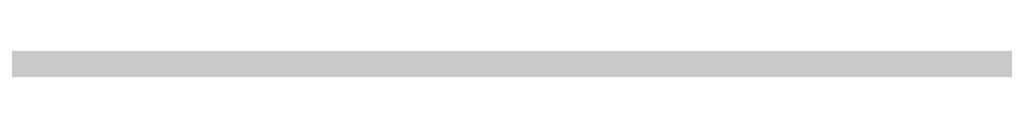
# Model space of a CAD drawing. Units: inches. Extents: x 2091 to 2899, y 967 to 2217.
# Tile 183 of 256: x 2203.16122 to 2203.18039, y 1152.24727 to 1152.24748. Entities that reach past the tile are written whole.
import ezdxf

# ---------------------------------------------------------------- set-up
doc = ezdxf.new("R2010")
doc.units = ezdxf.units.IN
doc.layers.add('A-WALL-PATT', color=141, linetype='Continuous', lineweight=13, true_color=0xadddf7)

msp = doc.modelspace()

# ---------------------------------------------------------------- hatches: boundary and pattern name
at = {"layer": 'A-WALL-PATT'}
h = msp.add_hatch(color=256, dxfattribs=at)
h.dxf.hatch_style = 1
h.paths.add_polyline_path([(2803.143603, 2050.919059), (2203.143603, 2050.919059), (2203.143603, 1090.919059), (2803.143603, 1090.919059)])
h.paths.add_polyline_path([(2635.79885, 1147.540465), (2674.524052, 1147.540465, 0.376086), (2678.529665, 1152.880202), (2678.529665, 1159.556473, 0.333335), (2674.524319, 1163.561846), (2674.524319, 1163.56185), (2674.524319, 1192.93439), (2635.805971, 1192.93439), (2597.087622, 1192.93439), (2597.087622, 1163.561846, 0.333335), (2593.082276, 1159.556473), (2593.082276, 1152.880202, 0.376086), (2597.087889, 1147.540465)], flags=0)
h.paths.add_polyline_path([(2436.010433, 1278.240778, 0.000483), (2435.952643, 1278.215027, -0.001328), (2435.935625, 1278.111693, -0.001711), (2436.11644, 1278.040758, 0.002185)], flags=0)
h.paths.add_polyline_path([(2794.143603, 1143.419059), (2794.143603, 1347.419059), (2543.370171, 1347.419059), (2543.370171, 1351.919059), (2794.143603, 1351.919059), (2794.143603, 1392.713555), (2793.947398, 1392.713555), (2793.947398, 1473.5369), (2794.143603, 1473.5369), (2794.143603, 1531.919059), (2650.143603, 1531.919059), (2650.143603, 1536.419059), (2794.143603, 1536.419059), (2794.143603, 1692.419059), (2609.375609, 1692.419059), (2609.375609, 1644.419059), (2604.875609, 1644.419059), (2604.875609, 1744.919059), (2609.375609, 1744.919059), (2609.375609, 1696.919059), (2794.143603, 1696.919059), (2794.143603, 1780.919059), (2609.643603, 1780.919059), (2493.875609, 1780.919059), (2493.875609, 1785.419059), (2609.643603, 1785.419059), (2794.143603, 1785.419059), (2794.143603, 1847.938821), (2793.951222, 1847.938821), (2793.951222, 1928.762166), (2794.143603, 1928.762166), (2794.143603, 1941.419059), (2614.143603, 1941.419059), (2614.143603, 1821.419059), (2609.643603, 1821.419059), (2609.643603, 1941.419059), (2392.143603, 1941.419059), (2392.143603, 1819.919059), (2387.643603, 1819.919059), (2387.643603, 1941.419059), (2212.143603, 1941.419059), (2212.143603, 1783.919059), (2392.143603, 1783.919059), (2392.143603, 1780.919059), (2212.143603, 1780.919059), (2212.143603, 1629.419059), (2387.643603, 1629.419059), (2387.643603, 1744.919059), (2392.143603, 1744.919059), (2392.143603, 1627.919059), (2317.143603, 1627.919059), (2317.143603, 1551.419059), (2317.143603, 1536.419059), (2459.383591, 1536.419059), (2459.383591, 1602.39648), (2463.883591, 1602.39648), (2463.883591, 1531.919059), (2456.643603, 1531.919059), (2456.643603, 1529.919059), (2452.143603, 1529.919059), (2452.143603, 1531.919059), (2312.643603, 1531.919059), (2312.643603, 1551.419059), (2306.143603, 1551.419059), (2306.143603, 1555.919059), (2308.143603, 1555.919059), (2308.143603, 1551.419059), (2312.643603, 1551.419059), (2312.643603, 1627.919059), (2212.143603, 1627.919059), (2212.143603, 1555.919059), (2270.143603, 1555.919059), (2270.143603, 1551.419059), (2212.143603, 1551.419059), (2212.143603, 1351.919059), (2272.143603, 1351.919059), (2272.143603, 1347.419059), (2212.143603, 1347.419059), (2212.143603, 1275.419059), (2308.143603, 1275.419059), (2308.143603, 1351.919059), (2452.143603, 1351.919059), (2452.143603, 1493.919059), (2456.643603, 1493.919059), (2456.643603, 1347.419059), (2312.643603, 1347.419059), (2312.643603, 1270.919059), (2212.143603, 1270.919059), (2212.143603, 1099.919059), (2281.237523, 1099.919059), (2282.871041, 1110.913803), (2282.008341, 1116.996603), (2278.557741, 1121.420403), (2268.205641, 1128.056203), (2272.087641, 1128.056203), (2273.812941, 1131.927003), (2279.420341, 1134.691903), (2285.027841, 1135.244903), (2287.615841, 1137.456803), (2288.047141, 1138.009803), (2289.341141, 1140.774703), (2291.066541, 1139.668703), (2292.360541, 1135.244903), (2295.379841, 1136.903803), (2296.242541, 1135.797903), (2297.105241, 1133.033003), (2300.124641, 1138.009803), (2303.143941, 1138.009803), (2304.437941, 1135.797903), (2303.143941, 1133.586003), (2306.594641, 1134.691903), (2307.888741, 1133.033003), (2310.908041, 1135.244903), (2313.927441, 1134.138903), (2315.62686, 1132.427102), (2308.320041, 1117.549603), (2290.203841, 1109.807903), (2288.909841, 1103.172103), (2289.272309, 1099.919059), (2434.918227, 1099.919059), (2431.593227, 1124.788059), (2429.930227, 1169.553059), (2430.927185, 1240.519694), (2435.658926, 1238.186126), (2437.135227, 1196.554059), (2438.798227, 1143.973059), (2442.678227, 1111.998059), (2446.558227, 1099.919059), (2794.143603, 1099.919059), (2794.143603, 1138.919059), (2548.032447, 1138.919059), (2548.032447, 1143.419059), (2548.032447, 1148.819059), (2546.668457, 1148.031559), (2528.685692, 1179.178622, 0.256256), (2512.032447, 1148.819059), (2512.032447, 1143.419059), (2512.032447, 1138.919059), (2507.532447, 1138.919059), (2507.532447, 1143.419059), (2507.532447, 1148.819059, 0.256256), (2490.879202, 1179.178622), (2472.896437, 1148.031559), (2471.532447, 1148.819059), (2471.532447, 1143.419059), (2467.032447, 1143.419059), (2467.032447, 1269.945786, 0.039061), (2460.909987, 1273.580059), (2467.032447, 1273.580059), (2467.032447, 1286.325364, 0.014511), (2465.216194, 1286.761905), (2467.032447, 1287.052576), (2467.032447, 1323.419059), (2471.532447, 1323.419059), (2471.532447, 1148.819059), (2489.532447, 1179.995973), (2490.896437, 1179.208473), (2490.879202, 1179.178622, -0.256256), (2507.532447, 1148.819059), (2507.532447, 1143.419059), (2512.032447, 1143.419059), (2512.032447, 1148.819059, -0.256256), (2528.685692, 1179.178622), (2528.668457, 1179.208473), (2530.032447, 1179.995973), (2548.032447, 1148.819059), (2548.032447, 1143.419059)], flags=16)
h.paths.add_polyline_path([(2607.768546, 1200.945083), (2607.768546, 1265.030625), (2597.087622, 1281.052011), (2619.784585, 1281.052011), (2627.795278, 1337.12686), (2635.79885, 1337.12686), (2643.816663, 1337.12686), (2651.827356, 1281.052011), (2674.524319, 1281.052011), (2663.843395, 1265.030625), (2663.843395, 1200.945083), (2635.805971, 1200.945083)], flags=0)
edge = h.paths.add_edge_path(flags=0)
edge.add_ellipse((13303.896215, 1272.998725), major_axis=(-10595.31304, 0.000001), ratio=0.842303870086, start_angle=0.6282372191, end_angle=0.6465540999, ccw=False)
edge.add_ellipse((2711.70045, 1156.852678), major_axis=(2.219769, 0), ratio=0.84230387, start_angle=111.535244, end_angle=180.628237, ccw=False)
edge.add_ellipse((13303.156292, 1272.998725), major_axis=(-10593.026306, 0), ratio=0.842303869544, start_angle=0.5282714718, end_angle=0.6465540971, ccw=False)
edge.add_line((2710.764596, 1175.333295), (2710.129986, 1175.333295))
edge.add_ellipse((2710.129986, 1176.579775), major_axis=(1.479846, 0), ratio=0.84230387, start_angle=180, end_angle=270, ccw=False)
edge.add_line((2708.65014, 1176.579775), (2708.65014, 1200.782914))
edge.add_ellipse((2710.129986, 1200.782914), major_axis=(1.479846, 0), ratio=0.84230387, start_angle=90, end_angle=180, ccw=False)
edge.add_line((2710.129986, 1202.029394), (2710.465075, 1202.029394))
edge.add_ellipse((13303.156292, 1272.998725), major_axis=(-10593.026306, 0), ratio=0.842303869544, start_angle=-0.0902290886, end_angle=0.3838667788, ccw=False)
edge.add_ellipse((2710.129986, 1290.927031), major_axis=(-1.479846, 0), ratio=0.84230387, start_angle=0, end_angle=90, ccw=False)
edge.add_line((2708.65014, 1290.927031), (2708.65014, 1315.13017))
edge.add_ellipse((2710.129986, 1315.13017), major_axis=(-1.479846, 0), ratio=0.84230387, start_angle=-90, end_angle=0, ccw=False)
edge.add_line((2710.129986, 1316.37665), (2710.706314, 1316.37665))
edge.add_ellipse((3238.40172, 1296.289566), major_axis=(528.234, 0), ratio=0.8423038695, start_angle=176.34957241, end_angle=177.82004969, ccw=False)
edge.add_ellipse((2775.063043, 1071.450696), major_axis=(313.307761, 0), ratio=0.8423038695, start_angle=102.12596555, end_angle=103.78052899, ccw=False)
edge.add_ellipse((2775.063043, 1078.305698), major_axis=(-305.302891, 0), ratio=0.8423038695, start_angle=-79.790461, end_angle=-77.55537271, ccw=False)
edge.add_ellipse((2695.141767, 1541.975383), major_axis=(-250.960216, 0), ratio=0.8423038695, start_angle=99.25656601, end_angle=102.55493264)
edge.add_line((2741.410326, 1334.214255), (2747.132545, 1337.378477))
edge.add_ellipse((2747.538616, 1336.857478), major_axis=(-0.739923, 0), ratio=0.8423039, start_angle=270, end_angle=307.93313, ccw=False)
edge.add_ellipse((2747.538616, 1336.857478), major_axis=(-0.739923, 0), ratio=0.8423039, start_angle=232.06687, end_angle=270, ccw=False)
edge.add_line((2747.944687, 1337.378477), (2753.666906, 1334.214255))
edge.add_ellipse((2799.935466, 1541.975383), major_axis=(250.960216, 0), ratio=0.8423038695, start_angle=257.44506736, end_angle=260.74343399)
edge.add_ellipse((2720.014189, 1078.305698), major_axis=(305.302891, 0), ratio=0.8423038695, start_angle=77.55537271, end_angle=79.790461, ccw=False)
edge.add_ellipse((2720.014189, 1071.450696), major_axis=(-313.307761, 0), ratio=0.8423038695, start_angle=256.21947101, end_angle=257.87403445, ccw=False)
edge.add_ellipse((2256.675512, 1296.289566), major_axis=(-528.234, 0), ratio=0.8423038695, start_angle=182.17995031, end_angle=183.65042759, ccw=False)
edge.add_line((2784.370918, 1316.37665), (2784.947247, 1316.37665))
edge.add_ellipse((2784.947247, 1315.13017), major_axis=(1.479846, 0), ratio=0.84230387, start_angle=0, end_angle=90, ccw=False)
edge.add_line((2786.427093, 1315.13017), (2786.427093, 1290.927031))
edge.add_ellipse((2784.947247, 1290.927031), major_axis=(1.479846, 0), ratio=0.84230387, start_angle=270, end_angle=360, ccw=False)
edge.add_ellipse((-7808.07906, 1272.998725), major_axis=(10593.026306, 0), ratio=0.842303869544, start_angle=-0.3838667788, end_angle=0.0902290886, ccw=False)
edge.add_line((2784.612157, 1202.029394), (2784.947247, 1202.029394))
edge.add_ellipse((2784.947247, 1200.782914), major_axis=(1.479846, 0), ratio=0.84230387, start_angle=0, end_angle=90, ccw=False)
edge.add_line((2786.427093, 1200.782914), (2786.427093, 1176.579775))
edge.add_ellipse((2784.947247, 1176.579775), major_axis=(-1.479846, 0), ratio=0.84230387, start_angle=90, end_angle=180, ccw=False)
edge.add_line((2784.947247, 1175.333295), (2784.312636, 1175.333295))
edge.add_ellipse((-7808.07906, 1272.998725), major_axis=(10593.026306, 0), ratio=0.842303869544, start_angle=-0.6186431963, end_angle=-0.5282714718, ccw=False)
edge.add_ellipse((2783.376783, 1156.852678), major_axis=(-2.219769, 0), ratio=0.84230387, start_angle=179.371763, end_angle=248.464757, ccw=False)
edge.add_ellipse((-7808.818983, 1272.998725), major_axis=(-10595.31304, 0.000004), ratio=0.842303865762, start_angle=179.3534459226, end_angle=179.3717628034, ccw=False)
edge.add_ellipse((2780.297303, 1153.500793), major_axis=(-5.246426, 0), ratio=0.84230387, start_angle=90, end_angle=179.353446, ccw=False)
edge.add_line((2780.297303, 1149.081708), (2714.77993, 1149.081708))
edge.add_ellipse((2714.77993, 1153.500793), major_axis=(5.246426, 0), ratio=0.84230387, start_angle=180.646554, end_angle=270, ccw=False)
edge = h.paths.add_edge_path(flags=0)
edge.add_line((2718.187367, 1151.007833), (2718.187367, 1170.472364))
edge.add_ellipse((2721.14706, 1170.472364), major_axis=(-2.959692, 0), ratio=0.84230387, start_angle=-90, end_angle=0, ccw=False)
edge.add_line((2721.14706, 1172.965324), (2773.930173, 1172.965324))
edge.add_ellipse((2773.930173, 1170.472364), major_axis=(-2.959692, 0), ratio=0.84230387, start_angle=180, end_angle=270, ccw=False)
edge.add_line((2776.889865, 1170.472364), (2776.889865, 1151.007833))
edge.add_line((2776.889865, 1151.007833), (2718.187367, 1151.007833))
edge = h.paths.add_edge_path(flags=0)
edge.add_line((2718.187367, 1180.23415), (2718.187367, 1199.057834))
edge.add_ellipse((2747.538616, 1320.39864), major_axis=(147.017924, 0), ratio=0.8423038695, start_angle=256.40186531, end_angle=283.59813469)
edge.add_line((2776.889865, 1199.057834), (2776.889865, 1180.23415))
edge.add_ellipse((2747.538616, 1301.574956), major_axis=(147.017924, 0), ratio=0.8423038695, start_angle=256.40186531, end_angle=283.59813469, ccw=False)
edge = h.paths.add_edge_path(flags=0)
edge.add_ellipse((13303.156292, 1272.998725), major_axis=(-10591.54646, 0), ratio=0.842303869555, start_angle=0.0555943135, end_angle=0.3777641939, ccw=False)
edge.add_line((2711.616859, 1262.72171), (2715.667408, 1249.495396))
edge.add_ellipse((6413.891963, 1241.691919), major_axis=(-3698.236159, 0), ratio=0.84230386955, start_angle=-0.120897369, end_angle=0.364076349)
edge.add_line((2715.761038, 1218.192455), (2711.934307, 1203.167361))
edge = h.paths.add_edge_path(flags=0)
edge.add_line((2718.187367, 1251.074566), (2716.002485, 1267.450435))
edge.add_ellipse((2742.151175, 1202.18954), major_axis=(81.772585, 0), ratio=0.84230387, start_angle=94.27742096, end_angle=111.8349538, ccw=False)
edge.add_line((2737.009748, 1270.930626), (2758.067484, 1270.930626))
edge.add_ellipse((2752.926058, 1202.18954), major_axis=(81.772585, 0), ratio=0.84230387, start_angle=68.1650462, end_angle=85.72257904, ccw=False)
edge.add_line((2779.074747, 1267.450435), (2776.889865, 1251.074566))
edge.add_ellipse((2750.338059, 1187.885356), major_axis=(79.579664, 0), ratio=0.84230387, start_angle=67.20808512, end_angle=85.1299304)
edge.add_line((2756.034656, 1254.743656), (2739.042576, 1254.743656))
edge.add_ellipse((2744.739174, 1187.885356), major_axis=(79.579664, 0), ratio=0.84230387, start_angle=94.8700696, end_angle=112.79191488)
edge = h.paths.add_edge_path(flags=0)
edge.add_line((2783.142926, 1203.167361), (2779.316194, 1218.192455))
edge.add_ellipse((-918.81473, 1241.691919), major_axis=(3698.236159, 0), ratio=0.84230386955, start_angle=-0.364076349, end_angle=0.120897369)
edge.add_line((2779.409825, 1249.495396), (2783.460373, 1262.72171))
edge.add_ellipse((-7808.07906, 1272.998725), major_axis=(-10591.54646, 0), ratio=0.84230386954, start_angle=179.6222358061, end_angle=179.9444056865, ccw=False)
edge = h.paths.add_edge_path(flags=0)
edge.add_ellipse((2734.200892, 1286.69044), major_axis=(-0.356609, 6.340078), ratio=0.60383358, start_angle=89.0020143, end_angle=253.657408, ccw=False)
edge.add_line((2730.369001, 1286.541806), (2730.369001, 1301.35198))
edge.add_line((2730.369001, 1301.35198), (2735.913311, 1305.214803))
edge.add_ellipse((2736.384917, 1304.734561), major_axis=(0.739923, 0), ratio=0.8423039, start_angle=90, end_angle=134.480211, ccw=False)
edge.add_line((2736.384917, 1305.357801), (2738.032783, 1305.357801))
edge.add_line((2738.032783, 1305.357801), (2738.032783, 1307.707927))
edge.add_ellipse((2794.201642, 1307.707927), major_axis=(56.168859, 0), ratio=0.84230387, start_angle=150.5614304, end_angle=180, ccw=False)
edge.add_ellipse((2700.875591, 1307.707927), major_axis=(-56.168859, 0), ratio=0.84230387, start_angle=180, end_angle=209.4385696, ccw=False)
edge.add_line((2757.04445, 1307.707927), (2757.04445, 1305.357801))
edge.add_line((2757.04445, 1305.357801), (2758.692316, 1305.357801))
edge.add_ellipse((2758.692316, 1304.734561), major_axis=(-0.739923, 0), ratio=0.8423039, start_angle=225.519789, end_angle=270, ccw=False)
edge.add_line((2759.163922, 1305.214803), (2764.708231, 1301.35198))
edge.add_line((2764.708231, 1301.35198), (2764.708231, 1286.541806))
edge.add_ellipse((2760.87634, 1286.69044), major_axis=(0.356609, 6.340078), ratio=0.60383358, start_angle=106.342592, end_angle=270.9979857, ccw=False)
edge.add_line((2757.04445, 1285.79709), (2757.04445, 1307.707927))
edge.add_ellipse((2700.875591, 1307.707927), major_axis=(-56.168859, 0), ratio=0.84230387, start_angle=180, end_angle=209.4385696)
edge.add_ellipse((2794.201642, 1307.707927), major_axis=(56.168859, 0), ratio=0.84230387, start_angle=150.5614304, end_angle=180)
edge.add_line((2738.032783, 1307.707927), (2738.032783, 1285.79709))
h.paths.add_polyline_path([(2417.812273, 1104.449704), (2413.492273, 1102.529704), (2410.612273, 1103.969704), (2409.172273, 1106.369704), (2407.252273, 1107.329704), (2406.292273, 1109.729704), (2405.332273, 1114.049704), (2405.332273, 1117.889704), (2406.292273, 1120.129704), (2407.252273, 1119.809704), (2408.848322, 1118.327658), (2410.173945, 1119.42417), (2410.211273, 1120.405704), (2411.040731, 1121.419054), (2410.699273, 1119.858704), (2410.173945, 1119.42417), (2410.088452, 1117.176109), (2411.132836, 1116.206324), (2413.972273, 1119.329704), (2416.852273, 1120.769704), (2416.869721, 1120.798784), (2417.035071, 1119.405116), (2417.896213, 1118.143384), (2418.292273, 1118.369704), (2419.544447, 1120.039269), (2419.360915, 1118.387487), (2419.032108, 1119.356151), (2418.398939, 1118.511926), (2419.252273, 1114.529704), (2418.794091, 1107.198795)], flags=0)
h.paths.add_polyline_path([(2508.870171, 1347.419059), (2508.370171, 1347.419059), (2508.370171, 1351.919059), (2508.870171, 1351.919059)], flags=0)
h.paths.add_polyline_path([(2473.370171, 1347.419059), (2472.370171, 1347.419059), (2467.870171, 1347.419059), (2467.870171, 1455.419059), (2472.370171, 1455.419059), (2472.370171, 1352.419059), (2473.370171, 1352.419059)], flags=0)
h.paths.add_polyline_path([(2352.106244, 1217.446197), (2349.226244, 1218.886197), (2347.786244, 1221.286197), (2345.866244, 1222.246197), (2344.906244, 1224.646197), (2343.946244, 1228.966197), (2343.946244, 1232.806197), (2344.906244, 1235.046197), (2345.866244, 1234.726197), (2347.462293, 1233.244152), (2348.787916, 1234.340663), (2348.825244, 1235.322197), (2349.654702, 1236.335547), (2349.313244, 1234.775197), (2348.787916, 1234.340663), (2348.702423, 1232.092603), (2349.746807, 1231.122817), (2352.586244, 1234.246197), (2355.466244, 1235.686197), (2355.483692, 1235.715277), (2355.649043, 1234.321609), (2356.510185, 1233.059877), (2356.906244, 1233.286197), (2358.158418, 1234.955762), (2357.974887, 1233.30398), (2357.646079, 1234.272644), (2357.012911, 1233.428419), (2357.866244, 1229.446197), (2357.408062, 1222.115288), (2356.426244, 1219.366197)], flags=0)
h.paths.add_polyline_path([(2348.2968, 1112.22442), (2347.0138, 1112.31042), (2345.5298, 1114.12742), (2345.7318, 1115.85842), (2346.8118, 1116.98242), (2346.8118, 1114.64642), (2345.8668, 1114.21442), (2346.8798, 1114.30042)], flags=0)
h.paths.add_polyline_path([(2347.0138, 1110.92642), (2346.2718, 1110.49342), (2346.6098, 1111.18642)], flags=0)
h.paths.add_polyline_path([(2345.8668, 1118.19442), (2345.5298, 1117.32942), (2343.7078, 1118.02142), (2344.3828, 1118.62642)], flags=0)
h.paths.add_polyline_path([(2346.6768, 1109.28242), (2346.0698, 1108.07142), (2345.8668, 1110.06142)], flags=0)
h.paths.add_polyline_path([(2345.0568, 1119.75142), (2343.6398, 1119.75142), (2343.9778, 1121.13542)], flags=0)
h.paths.add_polyline_path([(2345.2598, 1116.55042), (2345.1248, 1115.85842), (2344.9218, 1115.68542), (2344.7198, 1116.37742)], flags=0)
h.paths.add_polyline_path([(2345.6648, 1112.31042), (2345.4618, 1111.53242), (2344.0448, 1111.96442), (2344.6518, 1112.57042)], flags=0)
h.paths.add_polyline_path([(2345.1918, 1113.34942), (2344.4498, 1113.86842), (2344.7198, 1114.38742)], flags=0)
h.paths.add_polyline_path([(2344.6518, 1116.80942), (2344.1798, 1115.68542), (2344.6518, 1115.33942), (2343.9098, 1114.90642), (2343.0328, 1115.94442), (2343.6398, 1116.46342)], flags=0)
h.paths.add_polyline_path([(2345.8668, 1106.68642), (2344.9898, 1105.56242), (2344.5168, 1106.60042)], flags=0)
h.paths.add_polyline_path([(2344.8548, 1110.06142), (2344.5168, 1109.28242), (2344.1128, 1109.71542)], flags=0)
h.paths.add_polyline_path([(2344.0448, 1113.52242), (2343.4378, 1113.08942), (2342.7628, 1113.95442)], flags=0)
h.paths.add_polyline_path([(2344.3148, 1111.01242), (2342.9648, 1110.32042), (2342.9648, 1111.09942)], flags=0)
h.paths.add_polyline_path([(2345.1248, 1104.69742), (2344.5848, 1103.74542), (2344.4498, 1104.26442)], flags=0)
h.paths.add_polyline_path([(2342.8298, 1121.22242), (2341.7498, 1120.53042), (2340.5358, 1121.04942), (2340.1308, 1121.82842), (2340.6708, 1122.95242), (2341.1428, 1121.82842), (2341.6148, 1122.00142)], flags=0)
h.paths.add_polyline_path([(2342.9648, 1119.75142), (2343.0328, 1118.45342), (2342.0878, 1118.02142), (2342.0198, 1119.49142)], flags=0)
h.paths.add_polyline_path([(2342.6948, 1116.89642), (2341.9528, 1116.63642), (2342.0198, 1117.32942)], flags=0)
h.paths.add_polyline_path([(2343.0328, 1112.22442), (2342.0198, 1111.79142), (2341.5478, 1112.22442), (2342.3578, 1113.34942)], flags=0)
h.paths.add_polyline_path([(2343.7748, 1104.43742), (2342.6278, 1102.88042), (2342.6948, 1104.61042), (2343.4378, 1105.12942)], flags=0)
h.paths.add_polyline_path([(2342.0198, 1115.07942), (2340.8058, 1115.51242), (2340.9408, 1116.37742)], flags=0)
h.paths.add_polyline_path([(2341.4808, 1120.09742), (2341.4808, 1119.40542), (2341.0758, 1119.57842), (2341.1428, 1120.09742)], flags=0)
h.paths.add_polyline_path([(2341.8178, 1114.47342), (2340.9408, 1113.08942), (2340.8058, 1114.56042)], flags=0)
h.paths.add_polyline_path([(2341.1428, 1118.54042), (2340.9408, 1116.98242), (2339.0508, 1117.67542), (2339.0508, 1118.62642)], flags=0)
h.paths.add_polyline_path([(2342.6948, 1101.66842), (2341.9528, 1101.84142), (2342.5598, 1102.36142)], flags=0)
h.paths.add_polyline_path([(2340.3328, 1119.66542), (2338.4438, 1119.57842), (2337.9038, 1120.35742), (2339.6578, 1120.61642)], flags=0)
h.paths.add_polyline_path([(2340.3328, 1115.33942), (2340.0628, 1113.69542), (2339.3878, 1115.33942)], flags=0)
h.paths.add_polyline_path([(2341.8178, 1103.83142), (2341.5478, 1102.88042), (2341.1428, 1103.65842)], flags=0)
h.paths.add_polyline_path([(2339.0508, 1122.86642), (2337.2958, 1121.82842), (2337.0938, 1123.12542), (2337.7688, 1123.81842)], flags=0)
h.paths.add_polyline_path([(2339.1178, 1121.74142), (2338.8478, 1121.22242), (2338.1738, 1121.04942), (2338.3758, 1121.56842)], flags=0)
h.paths.add_polyline_path([(2339.1858, 1119.31942), (2338.6458, 1118.71342), (2338.2408, 1118.10742), (2338.2408, 1118.88642)], flags=0)
h.paths.add_polyline_path([(2341.1428, 1101.92842), (2340.6028, 1101.23642), (2340.0628, 1101.84142), (2340.6028, 1102.36142)], flags=0)
h.paths.add_polyline_path([(2337.6338, 1117.76142), (2336.6208, 1118.28042), (2337.2958, 1118.97242)], flags=0)
h.paths.add_polyline_path([(2336.8238, 1119.57842), (2334.7988, 1118.97242), (2335.2038, 1120.35742), (2336.5538, 1120.87642)], flags=0)
h.paths.add_polyline_path([(2339.1178, 1100.45742), (2337.3638, 1100.54342), (2336.7558, 1101.23642)], flags=0)
h.paths.add_polyline_path([(2336.3508, 1122.43342), (2336.0138, 1121.91442), (2334.9338, 1122.43342), (2334.5288, 1123.47142), (2335.7438, 1122.77942)], flags=0)
h.paths.add_polyline_path([(2334.7318, 1120.87642), (2334.2588, 1120.35742), (2334.0568, 1120.78942), (2334.5968, 1121.30842)], flags=0)
h.paths.add_polyline_path([(2334.4618, 1122.17442), (2332.5718, 1121.30842), (2331.3568, 1122.17442), (2332.0998, 1122.86642)], flags=0)
h.paths.add_polyline_path([(2334.2588, 1118.54042), (2333.3818, 1118.45342), (2333.6518, 1119.31942)], flags=0)
h.paths.add_polyline_path([(2335.5418, 1102.27442), (2334.1918, 1102.62042), (2335.2718, 1103.31242)], flags=0)
h.paths.add_polyline_path([(2332.7068, 1119.66542), (2331.6948, 1120.44342), (2332.5048, 1120.78942)], flags=0)
h.paths.add_polyline_path([(2334.7318, 1101.14942), (2333.5168, 1101.58242), (2333.9888, 1101.75542)], flags=0)
h.paths.add_polyline_path([(2332.6398, 1116.63642), (2331.0868, 1116.29042), (2331.9648, 1118.19442)], flags=0)
h.paths.add_polyline_path([(2330.7498, 1121.56842), (2330.2768, 1120.27042), (2328.5228, 1119.31942), (2328.9948, 1121.04942)], flags=0)
h.paths.add_polyline_path([(2330.7498, 1118.62642), (2330.0078, 1117.50242), (2329.8728, 1118.02142)], flags=0)
h.paths.add_polyline_path([(2332.0998, 1102.36142), (2330.5468, 1102.01442), (2331.6948, 1102.96642)], flags=0)
h.paths.add_polyline_path([(2329.5348, 1113.60842), (2329.0628, 1112.31042), (2328.5898, 1113.34942)], flags=0)
h.paths.add_polyline_path([(2328.3878, 1117.84842), (2327.5098, 1116.55042), (2327.1728, 1117.76142)], flags=0)
h.paths.add_polyline_path([(2329.7378, 1106.51342), (2329.5348, 1105.30242), (2328.2528, 1106.08142)], flags=0)
h.paths.add_polyline_path([(2328.6578, 1114.38742), (2328.0498, 1114.12742), (2328.3198, 1114.90642)], flags=0)
h.paths.add_polyline_path([(2328.3198, 1112.22442), (2327.1058, 1112.13742), (2326.7008, 1112.65642)], flags=0)
h.paths.add_polyline_path([(2326.9028, 1115.25242), (2326.7008, 1114.12742), (2325.2158, 1113.60842), (2326.0928, 1115.33942)], flags=0)
h.paths.add_polyline_path([(2326.6328, 1108.33042), (2326.0928, 1107.37942), (2325.8908, 1108.50342), (2326.4978, 1109.10942)], flags=0)
h.paths.add_polyline_path([(2615.143603, 1531.919059), (2609.643603, 1531.919059), (2609.643603, 1620.419059), (2614.143603, 1620.419059), (2614.143603, 1536.419059), (2615.143603, 1536.419059)], flags=0)
h.paths.add_polyline_path([(2545.143603, 1563.419059), (2464.143603, 1563.419059), (2464.143603, 1632.419059), (2509.143603, 1632.419059), (2509.143603, 1627.919059), (2509.143603, 1603.919059), (2468.643603, 1603.919059), (2468.643603, 1567.919059), (2540.643603, 1567.919059), (2540.643603, 1591.919059), (2545.143603, 1591.919059)], flags=0)
h.paths.add_polyline_path([(2388.969048, 1549.985735), (2357.434181, 1549.985735), (2357.434181, 1623.360778), (2399.362777, 1623.360778), (2435.689465, 1623.360778), (2435.592547, 1602.559273), (2435.592547, 1602.39648), (2388.969048, 1602.39648)], flags=0)
h.paths.add_polyline_path([(2388.880628, 1555.809151), (2374.904429, 1555.809151), (2374.904429, 1600.571564), (2374.904429, 1615.457645), (2406.350877, 1615.457645), (2406.350877, 1618.939431), (2412.174293, 1615.457645), (2406.350877, 1611.97586), (2406.350877, 1615.457645), (2388.880628, 1615.457645)], flags=0)
h.paths.add_polyline_path([(2568.875609, 1644.419059), (2453.375609, 1644.419059), (2453.375609, 1785.419059), (2457.875609, 1785.419059), (2457.875609, 1648.919059), (2568.875609, 1648.919059)], flags=0)
h.paths.add_polyline_path([(2212.143603, 1945.919059), (2212.143603, 2041.919059), (2794.143603, 2041.919059), (2794.143603, 1945.919059)], flags=16)
h.paths.add_polyline_path([(2271.082728, 1964.317238), (2776.852968, 1964.317238), (2776.852968, 2037.169623), (2271.082728, 2037.169623)], flags=8)
h.paths.add_polyline_path([(2380.649285, 1536.824144), (2461.040809, 1536.824144), (2461.040809, 1554.652587), (2380.649285, 1554.652587)], flags=8)
h.paths.add_polyline_path([(2240.755709, 1609.725451), (2309.185829, 1609.725451), (2309.185829, 1617.698204), (2240.755709, 1617.698204)], flags=8)
h.paths.add_polyline_path([(2212.677255, 1313.504102), (2282.59152, 1313.504102), (2282.59152, 1322.745239), (2212.677255, 1322.745239)], flags=8)
h.paths.add_polyline_path([(2457.111976, 1114.778574), (2558.481581, 1114.778574), (2558.481581, 1142.219682), (2457.111976, 1142.219682)], flags=8)
h.paths.add_polyline_path([(2473.442337, 1273.010067), (2604.641226, 1273.010067), (2604.641226, 1318.346935), (2473.442337, 1318.346935)], flags=8)
h.paths.add_polyline_path([(2638.876302, 1626.977432), (2684.250367, 1627.976738), (2684.038483, 1637.597494), (2638.664417, 1636.598188)], flags=8)
h.paths.add_polyline_path([(2537.590554, 1453.793447), (2628.389547, 1453.793447), (2628.389547, 1475.344811), (2537.590554, 1475.344811)], flags=8)
h.paths.add_polyline_path([(2504.137638, 1714.632397), (2554.647187, 1714.632397), (2554.647187, 1730.237712), (2504.137638, 1730.237712)], flags=8)
h.paths.add_polyline_path([(2487.501181, 1575.651872), (2535.097121, 1575.651872), (2535.097121, 1598.377646), (2487.501181, 1598.377646)], flags=8)
h.paths.add_polyline_path([(2709.0994, 1735.710278), (2740.016601, 1735.710278), (2740.016601, 1749.937641), (2709.0994, 1749.937641)], flags=8)
h.paths.add_polyline_path([(2442.438424, 1792.171657), (2564.728835, 1792.171657), (2564.728835, 1842.000163), (2442.438424, 1842.000163)], flags=8)
h.paths.add_polyline_path([(2655.815801, 1809.644076), (2789.520142, 1806.693796), (2790.084977, 1832.291638), (2656.380635, 1835.241918)], flags=8)
h.paths.add_polyline_path([(2234.842697, 1797.720143), (2368.592851, 1794.768852), (2369.160718, 1820.504132), (2235.410564, 1823.455423)], flags=8)
h.paths.add_polyline_path([(2245.138466, 1644.006335), (2398.427733, 1640.6239), (2398.994842, 1666.32482), (2245.705575, 1669.707255)], flags=8)
h.paths.add_polyline_path([(2306.142847, 1431.168519), (2413.768314, 1428.793687), (2414.333148, 1454.391529), (2306.707682, 1456.76636)], flags=8)
h.paths.add_polyline_path([(2306.834582, 1458.233145), (2393.380484, 1456.323449), (2393.932808, 1481.354358), (2307.386907, 1483.264054)], flags=8)

doc.saveas('drawing.dxf')
